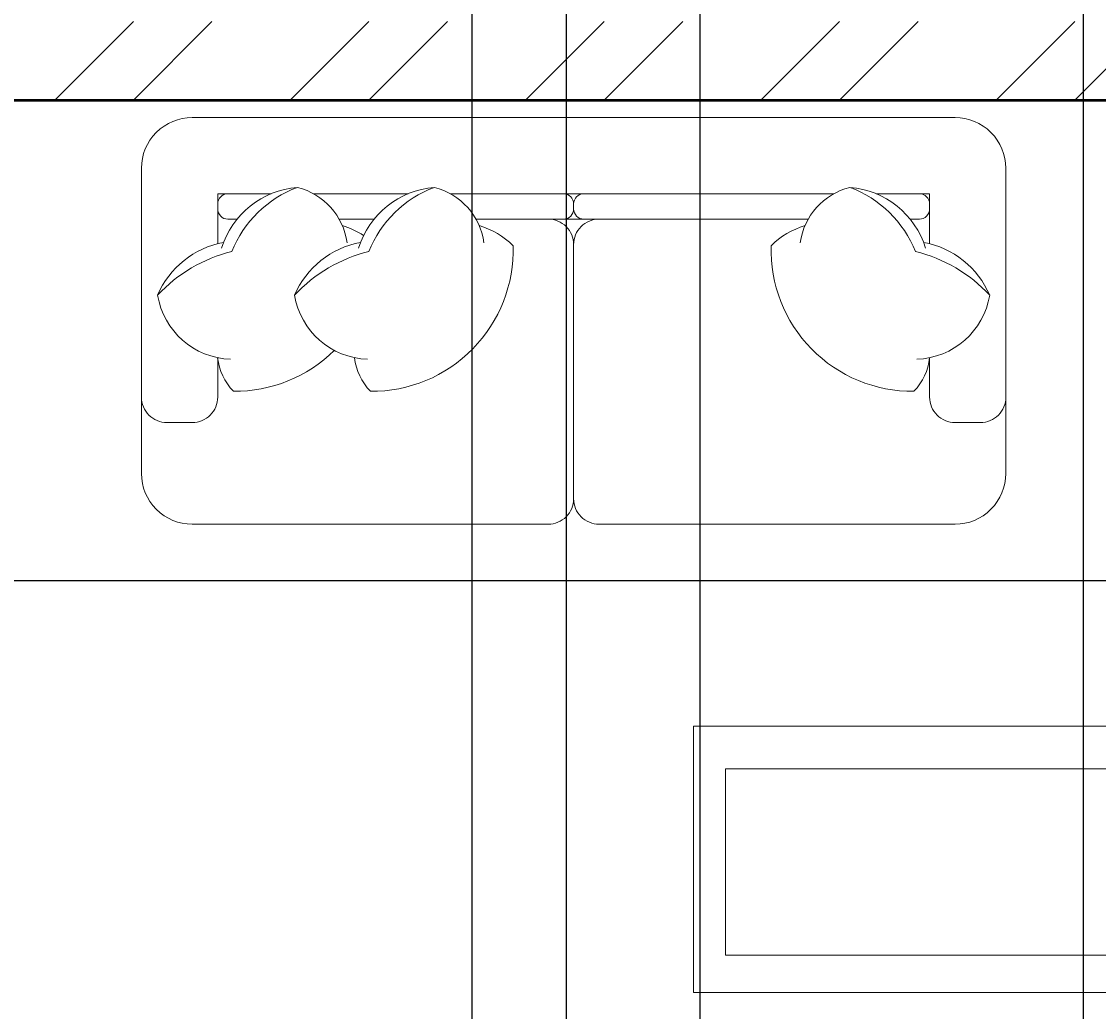
# Model space of a CAD drawing. Units: inches. Extents: x 2310 to 2937, y 1113 to 2410.
# Tile 5 of 23: x 2411 to 2472, y 1943 to 2000. Entities that reach past the tile are written whole.
import ezdxf

# ---------------------------------------------------------------- set-up
doc = ezdxf.new("R2010")
doc.units = ezdxf.units.IN
for name, color, linetype, lineweight in [('A-ANNO-DIMS', 2, 'Continuous', 18), ('A-FURN', 8, 'Continuous', 18), ('A-WALL', 7, 'Continuous', 50), ('A-WALL-PATT', 85, 'Continuous', 13)]:
    doc.layers.add(name, color=color, linetype=linetype, lineweight=lineweight)
doc.styles.get("Standard").update_dxf_attribs({"font": 'arial.ttf'})
doc.dimstyles.get("Standard").update_dxf_attribs({"dimtxt": 0.18, "dimasz": 0.18, "dimexe": 0.18, "dimexo": 0.0625, "dimgap": 0.09, "dimtad": 0, "dimtih": 1, "dimtoh": 1, "dimdec": 4, "dimzin": 0, "dimdsep": 46, "dimtxsty": 'Standard', "dimcen": 0.09, "dimadec": 0, "dimazin": 0, "dimtfac": 1, "dimtdec": 4, "dimtofl": 0, "dimtmove": 0, "dimatfit": 3, "dimfxl": 1, "dimtolj": 1, "dimtzin": 0, "dimarcsym": 0})

# ---------------------------------------------------------------- blocks, each defined once
blk = doc.blocks.new('*D57')
at = {"layer": 'A-ANNO-DIMS', "color": 0, "lineweight": -2, "transparency": 16777216}
for p, q in [((2403.548, 1995.014), (2858.016, 1995.014)), ((2857.836, 1994.834), (2857.836, 1981.45)), ((2857.836, 1967.702), (2857.836, 1981.086)), ((2403.548, 1967.522), (2858.016, 1967.522))]:
    blk.add_line(p, q, dxfattribs=at)
at = {"layer": 'A-ANNO-DIMS', "color": 0, "transparency": 16777216}
for points in [[(2857.806, 1994.834), (2857.866, 1994.834), (2857.836, 1995.014)], [(2857.806, 1967.702), (2857.866, 1967.702), (2857.836, 1967.522)]]:
    blk.add_solid(points, dxfattribs=at)
at = {"layer": 'Defpoints', "color": 0, "transparency": 16777216}
for p in [(2403.486, 1995.014), (2403.486, 1967.522), (2857.836, 1967.522)]:
    blk.add_point(p, dxfattribs=at)
at = {"layer": 'A-ANNO-DIMS', "color": 0, "transparency": 16777216, "insert": (2857.836, 1981.268), "char_height": 0.18, "attachment_point": 5}
blk.add_mtext('\\A1;27.49', dxfattribs=at)
blk = doc.blocks.new('*D60')
at = {"layer": 'A-ANNO-DIMS', "color": 0, "lineweight": -2, "transparency": 16777216}
for p, q in [((2449.502, 2205.951), (2449.502, 1649.501)), ((2471.439, 2205.951), (2471.439, 1649.501)), ((2449.682, 1649.681), (2460.005, 1649.681)), ((2471.259, 1649.681), (2460.936, 1649.681))]:
    blk.add_line(p, q, dxfattribs=at)
at = {"layer": 'A-ANNO-DIMS', "color": 0, "transparency": 16777216}
for points in [[(2449.682, 1649.711), (2449.682, 1649.651), (2449.502, 1649.681)], [(2471.259, 1649.711), (2471.259, 1649.651), (2471.439, 1649.681)]]:
    blk.add_solid(points, dxfattribs=at)
at = {"layer": 'Defpoints', "color": 0, "transparency": 16777216}
for p in [(2449.502, 2206.014), (2471.439, 2206.014), (2471.439, 1649.681)]:
    blk.add_point(p, dxfattribs=at)
at = {"layer": 'A-ANNO-DIMS', "color": 0, "transparency": 16777216, "insert": (2460.471, 1649.681), "char_height": 0.18, "attachment_point": 5}
blk.add_mtext('\\A1;21.936', dxfattribs=at)
blk = doc.blocks.new('*D63')
at = {"layer": 'A-ANNO-DIMS', "color": 0, "lineweight": -2, "transparency": 16777216}
for p, q in [((2436.465, 1999.451), (2436.465, 1649.501)), ((2524.465, 1999.451), (2524.465, 1649.501)), ((2436.645, 1649.681), (2480.245, 1649.681)), ((2524.285, 1649.681), (2480.684, 1649.681))]:
    blk.add_line(p, q, dxfattribs=at)
at = {"layer": 'A-ANNO-DIMS', "color": 0, "transparency": 16777216}
for points in [[(2436.645, 1649.711), (2436.645, 1649.651), (2436.465, 1649.681)], [(2524.285, 1649.711), (2524.285, 1649.651), (2524.465, 1649.681)]]:
    blk.add_solid(points, dxfattribs=at)
at = {"layer": 'Defpoints', "color": 0, "transparency": 16777216}
for p in [(2436.465, 1999.514), (2524.465, 1999.514), (2524.465, 1649.681)]:
    blk.add_point(p, dxfattribs=at)
at = {"layer": 'A-ANNO-DIMS', "color": 0, "transparency": 16777216, "insert": (2480.465, 1649.681), "char_height": 0.18, "attachment_point": 5}
blk.add_mtext('\\A1;88', dxfattribs=at)
blk = doc.blocks.new('*D65')
at = {"layer": 'A-ANNO-DIMS', "color": 0, "lineweight": -2, "transparency": 16777216}
for p, q in [((2403.486, 2093.451), (2403.486, 1649.501)), ((2436.465, 2093.451), (2436.465, 1649.501)), ((2403.666, 1649.681), (2419.581, 1649.681)), ((2436.285, 1649.681), (2420.369, 1649.681))]:
    blk.add_line(p, q, dxfattribs=at)
at = {"layer": 'A-ANNO-DIMS', "color": 0, "transparency": 16777216}
for points in [[(2403.666, 1649.711), (2403.666, 1649.651), (2403.486, 1649.681)], [(2436.285, 1649.711), (2436.285, 1649.651), (2436.465, 1649.681)]]:
    blk.add_solid(points, dxfattribs=at)
at = {"layer": 'Defpoints', "color": 0, "transparency": 16777216}
for p in [(2403.486, 2093.514), (2436.465, 2093.514), (2436.465, 1649.681)]:
    blk.add_point(p, dxfattribs=at)
at = {"layer": 'A-ANNO-DIMS', "color": 0, "transparency": 16777216, "insert": (2419.975, 1649.681), "char_height": 0.18, "attachment_point": 5}
blk.add_mtext('\\A1;32.98', dxfattribs=at)
blk = doc.blocks.new('*D69')
at = {"layer": 'A-ANNO-DIMS', "color": 0, "lineweight": -2, "transparency": 16777216}
for p, q in [((2441.861, 2131.962), (2441.861, 1649.501)), ((2475.893, 2131.962), (2475.893, 1649.501)), ((2442.041, 1649.681), (2458.483, 1649.681)), ((2475.713, 1649.681), (2459.271, 1649.681))]:
    blk.add_line(p, q, dxfattribs=at)
at = {"layer": 'A-ANNO-DIMS', "color": 0, "transparency": 16777216}
for points in [[(2442.041, 1649.711), (2442.041, 1649.651), (2441.861, 1649.681)], [(2475.713, 1649.711), (2475.713, 1649.651), (2475.893, 1649.681)]]:
    blk.add_solid(points, dxfattribs=at)
at = {"layer": 'Defpoints', "color": 0, "transparency": 16777216}
for p in [(2441.861, 2132.024), (2475.893, 2132.024), (2475.893, 1649.681)]:
    blk.add_point(p, dxfattribs=at)
at = {"layer": 'A-ANNO-DIMS', "color": 0, "transparency": 16777216, "insert": (2458.877, 1649.681), "char_height": 0.18, "attachment_point": 5}
blk.add_mtext('\\A1;34.03', dxfattribs=at)

msp = doc.modelspace()

# ---------------------------------------------------------------- hatches: boundary and pattern name
at = {"layer": 'A-WALL-PATT'}
h = msp.add_hatch(dxfattribs=at)
h.set_pattern_fill('ANSI32', color=256)
h.paths.add_polyline_path([(2639.1394, 2356.5139), (2563.662, 2356.5139), (2563.662, 2347.5139), (2606.9859, 2347.5139), (2606.9859, 2210.5139), (2514.2692, 2210.5139), (2514.2692, 2206.0139), (2606.9859, 2206.0139), (2606.9859, 2098.0139), (2602.689, 2098.0139), (2602.689, 2093.5139), (2615.5262, 2093.5139), (2615.5262, 2095.7639), (2615.5262, 2098.0139), (2611.4859, 2098.0139), (2611.4859, 2206.0139), (2703.9391, 2206.0139), (2703.9391, 2208.2639), (2703.9391, 2210.5139), (2611.4859, 2210.5139), (2611.4859, 2347.5139), (2639.1394, 2347.5139)])
h.paths.add_polyline_path([(2823.9859, 2356.5139), (2699.1394, 2356.5139), (2699.1394, 2347.5139), (2738.4859, 2347.5139), (2738.4859, 2343.9266), (2742.9859, 2343.9266), (2742.9859, 2347.5139), (2814.9859, 2347.5139), (2814.9859, 2336.76), (2823.9859, 2336.76)])
h.paths.add_polyline_path([(2823.9859, 2312.76), (2814.9859, 2312.76), (2814.9859, 2299.5139), (2742.9859, 2299.5139), (2742.9859, 2323.0159), (2740.7359, 2323.0159), (2738.4859, 2323.0159), (2738.4859, 2210.5139), (2734.5483, 2210.5139), (2734.5483, 2206.0139), (2746.8769, 2206.0139), (2746.8769, 2208.2639), (2746.8769, 2210.5139), (2742.9859, 2210.5139), (2742.9859, 2295.0139), (2814.9859, 2295.0139), (2814.9859, 2269.8977), (2823.9859, 2269.8977)])
h.paths.add_polyline_path([(2823.9859, 2210.5139), (2823.9859, 2233.8977), (2819.4859, 2233.8977), (2814.9859, 2233.8977), (2814.9859, 2210.5139), (2769.9745, 2210.5139), (2769.9745, 2206.0139), (2814.9859, 2206.0139), (2814.9859, 2178.3027), (2823.9859, 2178.3027)])
h.paths.add_polyline_path([(2823.9859, 2118.3027), (2819.4859, 2118.3027), (2814.9859, 2118.3027), (2814.9859, 2098.0139), (2647.0333, 2098.0139), (2647.0333, 2093.5139), (2814.9859, 2093.5139), (2814.9859, 1999.5139), (2650.6052, 1999.5139), (2650.6052, 1995.0139), (2814.9859, 1995.0139), (2814.9859, 1969.9784), (2823.9859, 1969.9784)])
h.paths.add_polyline_path([(2403.4859, 2093.5139), (2569.9888, 2093.5139), (2569.9888, 2095.7639), (2569.9888, 2098.0139), (2403.4859, 2098.0139), (2403.4859, 2131.7587), (2394.4859, 2131.7587), (2394.4859, 1967.522), (2403.4859, 1967.522), (2403.4859, 1995.0139), (2569.8903, 1995.0139), (2569.8903, 1997.2639), (2569.8903, 1999.5139), (2403.4859, 1999.5139)])
h.paths.add_polyline_path([(2503.662, 2356.5139), (2394.4859, 2356.5139), (2394.4859, 2337.9231), (2398.9859, 2337.9231), (2403.4859, 2337.9231), (2403.4859, 2347.5139), (2475.4859, 2347.5139), (2475.4859, 2343.0384), (2479.9859, 2343.0384), (2479.9859, 2347.5139), (2503.662, 2347.5139)])
h.paths.add_polyline_path([(2498.3065, 1745.5139), (2479.9859, 1745.5139), (2479.9859, 1749.1663), (2477.7359, 1749.1663), (2475.4859, 1749.1663), (2475.4859, 1745.5139), (2403.4859, 1745.5139), (2403.4859, 1753.6409), (2398.9859, 1753.6409), (2394.4859, 1753.6409), (2394.4859, 1736.5139), (2498.3065, 1736.5139), (2498.3065, 1741.0139)])
h.paths.add_polyline_path([(2479.9859, 1882.5139), (2483.9367, 1882.5139), (2483.9367, 1887.0139), (2471.5501, 1887.0139), (2471.5501, 1885.1969), (2471.5501, 1882.5139), (2475.4859, 1882.5139), (2475.4859, 1798.0139), (2403.4859, 1798.0139), (2403.4859, 1828.0433), (2402.2852, 1828.0433), (2394.4859, 1828.0433), (2394.4859, 1777.6409), (2403.4859, 1777.6409), (2403.4859, 1793.5139), (2475.4859, 1793.5139), (2475.4859, 1769.1696), (2479.9859, 1769.1696)])
h.paths.add_polyline_path([(2403.4859, 1907.522), (2398.9859, 1907.522), (2394.4859, 1907.522), (2394.4859, 1864.0433), (2403.4859, 1864.0433), (2403.4859, 1882.5139), (2448.9325, 1882.5139), (2448.9325, 1884.7639), (2448.9325, 1887.0139), (2403.4859, 1887.0139)])
h.paths.add_polyline_path([(2702.2061, 1887.0139), (2611.4859, 1887.0139), (2611.4859, 1995.0139), (2615.6132, 1995.0139), (2615.6132, 1999.5139), (2602.4798, 1999.5139), (2602.4798, 1997.2639), (2602.4798, 1995.0139), (2606.9859, 1995.0139), (2606.9859, 1887.0139), (2516.2443, 1887.0139), (2516.2443, 1884.7639), (2516.2443, 1882.5139), (2606.9859, 1882.5139), (2606.9859, 1745.5139), (2558.3065, 1745.5139), (2558.3065, 1736.5139), (2638.8921, 1736.5139), (2638.8921, 1741.0139), (2638.8921, 1745.5139), (2611.4859, 1745.5139), (2611.4859, 1882.5139), (2702.2061, 1882.5139)])
h.paths.add_polyline_path([(2823.9859, 1909.9784), (2819.4859, 1909.9784), (2814.9859, 1909.9784), (2814.9859, 1887.0139), (2769.144, 1887.0139), (2769.144, 1884.7639), (2769.144, 1882.5139), (2814.9859, 1882.5139), (2814.9859, 1854.1704), (2823.9859, 1854.1704)])
h.paths.add_polyline_path([(2823.9859, 1818.1704), (2819.4859, 1818.1704), (2814.9859, 1818.1704), (2814.9859, 1798.0139), (2742.9859, 1798.0139), (2742.9859, 1882.5139), (2746.805, 1882.5139), (2746.805, 1887.0139), (2733.7334, 1887.0139), (2733.7334, 1884.7639), (2733.7334, 1882.5139), (2738.4859, 1882.5139), (2738.4859, 1771.1728), (2740.7359, 1771.1728), (2742.9859, 1771.1728), (2742.9859, 1793.5139), (2814.9859, 1793.5139), (2814.9859, 1783.6684), (2823.9859, 1783.6684)])
h.paths.add_polyline_path([(2823.9859, 1759.6684), (2814.9859, 1759.6684), (2814.9859, 1745.5139), (2742.9859, 1745.5139), (2742.9859, 1748.9831), (2740.7359, 1748.9831), (2738.4859, 1748.9831), (2738.4859, 1745.5139), (2698.8921, 1745.5139), (2698.8921, 1736.5139), (2823.9859, 1736.5139)])

# ---------------------------------------------------------------- linework, layer by layer
at = {"layer": 'A-FURN', "ltscale": 0.03}
msp.add_lwpolyline([(2443.7406, 1970.7383, -0.4142136), (2442.2854, 1972.1935, -0.4142136), (2440.8302, 1970.7383), (2420.4576, 1970.7383, -0.4142136), (2417.5472, 1973.6487), (2417.5472, 1991.1109, -0.4142136), (2420.4576, 1994.0213), (2464.1132, 1994.0213, -0.4142136), (2467.0236, 1991.1109), (2467.0236, 1973.6487, -0.4142136), (2464.1132, 1970.7383), (2443.7406, 1970.7383, -0.4142136), (2442.2854, 1972.1935, -0.4142136), (2440.8302, 1970.7383)], format="xyb", dxfattribs=at)
at = {"layer": 'A-FURN'}
for points in [[(2418.4733, 1983.8487, -0.1477299), (2422.7264, 1986.3496, -0.2133428), (2426.4792, 1990.0176, -0.1786618)], [(2422.1389, 1986.5489, -0.3066635), (2426.4792, 1990.0176, -0.30633), (2429.3146, 1986.8498, 0.8728472)], [(2426.3124, 1983.8487, -0.1477299), (2430.5655, 1986.3496, -0.2133428), (2434.3182, 1990.0176, -0.1786618)], [(2429.9779, 1986.5489, -0.3066635), (2434.3182, 1990.0176, -0.30633), (2437.1536, 1986.8498, 0.8728472)], [(2462.432, 1986.5489, 0.3066635), (2458.0917, 1990.0176, 0.30633), (2455.2563, 1986.8498, -0.8728472)], [(2466.0975, 1983.8487, 0.1477299), (2461.8444, 1986.3496, 0.2133428), (2458.0917, 1990.0176, 0.1786618)], [(2424.9741, 1989.6557), (2421.9128, 1989.6557), (2421.9128, 1986.7959, -0.4142136)], [(2423.0232, 1988.2005), (2422.4948, 1988.2005, -0.4142136), (2421.9128, 1988.7826), (2421.9128, 1989.0737, -0.4142136), (2422.4948, 1989.6557)], [(2422.4948, 1989.6557), (2424.9741, 1989.6557, -0.4142136)], [(2427.395, 1989.6557), (2432.8131, 1989.6557, -0.4142136)], [(2435.234, 1989.6557), (2441.7033, 1989.6557, -0.4142136), (2442.2854, 1989.0737), (2442.2854, 1988.7826, -0.4142136), (2441.7033, 1988.2005), (2436.6993, 1988.2005, -0.4142136)], [(2457.1758, 1989.6557), (2442.8675, 1989.6557, 0.4142136), (2442.2854, 1989.0737), (2442.2854, 1988.7826, 0.4142136), (2442.8675, 1988.2005), (2455.7105, 1988.2005, 0.4142136)], [(2462.076, 1989.6557), (2459.5967, 1989.6557, 0.4142136)], [(2461.5476, 1988.2005), (2462.076, 1988.2005, 0.4142136), (2462.6581, 1988.7826), (2462.6581, 1989.0737, 0.4142136), (2462.076, 1989.6557)], [(2430.8623, 1988.2005), (2428.8603, 1988.2005, -0.4142136)], [(2440.8302, 1988.2005, -0.4142136), (2442.2854, 1986.7454)], [(2440.8302, 1988.2005, -0.4142136), (2442.2854, 1986.7454), (2442.2854, 1972.1935, -0.4142136)], [(2443.7406, 1988.2005, 0.4142136), (2442.2854, 1986.7454)], [(2443.7406, 1988.2005, 0.4142136), (2442.2854, 1986.7454), (2442.2854, 1972.1935, 0.4142136)], [(2430.2624, 1987.2632, 0.0718654), (2429.0424, 1987.8321, -7.1154643)], [(2429.7486, 1980.2695, 0.1655406), (2430.6489, 1978.3468, 0.4259892), (2438.8215, 1986.6831, 0.1215233), (2436.8815, 1987.8321, -7.1154643)], [(2462.6612, 1980.2695, -0.1655406), (2461.761, 1978.3468, -0.4259892), (2453.5884, 1986.6831, -0.1215233), (2455.5284, 1987.8321, 7.1154643)], [(2422.643, 1980.1808, -0.3567724), (2418.4733, 1983.8487, -0.2495421), (2422.2515, 1986.8715, 9.6168803)], [(2430.4821, 1980.1808, -0.3567724), (2426.3124, 1983.8487, -0.2495421), (2430.0905, 1986.8715, 9.6168803)], [(2461.9278, 1980.1808, 0.3567724), (2466.0975, 1983.8487, 0.2495421), (2462.3194, 1986.8715, -9.6168803)], [(2421.9096, 1980.2695, 0.1655406), (2422.8098, 1978.3468, 0.2002311), (2428.5864, 1980.6885, 0.1215233)], [(2421.9128, 1980.2688), (2421.9128, 1978.0142, -0.4142136), (2420.4576, 1976.559), (2419.0024, 1976.559, -0.4142136), (2417.5472, 1978.0142)], [(2467.0236, 1978.0142, -0.4142136), (2465.5684, 1976.559), (2464.1132, 1976.559, -0.4142136), (2462.6581, 1978.0142), (2462.6581, 1980.2688)]]:
    msp.add_lwpolyline(points, format="xyb", dxfattribs=at)
for points in [[(2432.8131, 1989.6557), (2427.395, 1989.6557)], [(2457.1758, 1989.6557), (2435.234, 1989.6557)], [(2462.6581, 1986.7959), (2462.6581, 1989.6557), (2459.5967, 1989.6557)]]:
    msp.add_lwpolyline(points, dxfattribs=at)
msp.add_lwpolyline([(2442.8675, 1989.6557), (2441.7033, 1989.6557, -0.4142136), (2442.2854, 1989.0737), (2442.2854, 1988.7826, -0.4142136), (2441.7033, 1988.2005), (2442.8675, 1988.2005, -0.4142136), (2442.2854, 1988.7826), (2442.2854, 1989.0737, -0.4142136)], format="xyb", close=True, dxfattribs=at)
for points in [[(2449.1475, 1959.1855), (2483.1791, 1959.1855), (2483.1791, 1943.9281), (2449.1475, 1943.9281)], [(2450.9745, 1956.7439), (2481.2801, 1956.7439), (2481.2801, 1946.0624), (2450.9745, 1946.0624)]]:
    msp.add_lwpolyline(points, close=True, dxfattribs=at)
at = {"layer": 'A-WALL'}
msp.add_line((2403.4859, 1995.0139), (2571.4589, 1995.0139), dxfattribs=at)

# ---------------------------------------------------------------- dimensions: what is measured, and where the dimension line sits
at = {"layer": 'A-ANNO-DIMS'}
for base, p1, p2, override, picture, middle in [((2471.4388, 1649.6807), (2449.5024, 2206.0139), (2471.4388, 2206.0139), {"dimdec": 3, "dimlfac": 1, "dimrnd": 0, "dimzin": 0, "dimdsep": 46, "dimlunit": 2}, '*D60', (2460.4706, 1649.6807)), ((2475.8929, 1649.6807), (2441.8613, 2132.0241), (2475.8929, 2132.0241), {"dimdec": 2, "dimlfac": 1, "dimrnd": 0, "dimzin": 0, "dimdsep": 46, "dimlunit": 2}, '*D69', (2458.8771, 1649.6807)), ((2436.4647, 1649.6807), (2403.4859, 2093.5139), (2436.4647, 2093.5139), {"dimdec": 2, "dimlfac": 1, "dimrnd": 0, "dimzin": 0, "dimdsep": 46, "dimlunit": 2}, '*D65', (2419.9753, 1649.6807)), ((2524.4647, 1649.6807), (2436.4647, 1999.5139), (2524.4647, 1999.5139), {"dimdec": 0, "dimlfac": 1, "dimrnd": 0, "dimzin": 0, "dimdsep": 46, "dimlunit": 2}, '*D63', (2480.4647, 1649.6807))]:
    dim = msp.add_linear_dim(base=base, p1=p1, p2=p2, dimstyle='Standard', override=override, dxfattribs=at)
    dim.commit()
    dim.dimension.update_dxf_attribs({"geometry": picture, "text_midpoint": middle})
dim = msp.add_linear_dim(base=(2857.8359, 1967.522), p1=(2403.4859, 1995.0139), p2=(2403.4859, 1967.522), angle=90, dimstyle='Standard', override={"dimdec": 2, "dimlfac": 1, "dimrnd": 0, "dimzin": 0, "dimdsep": 46, "dimlunit": 2}, dxfattribs=at)
dim.commit()
dim.dimension.update_dxf_attribs({"geometry": '*D57', "text_midpoint": (2857.8359, 1981.268)})

doc.saveas('drawing.dxf')
